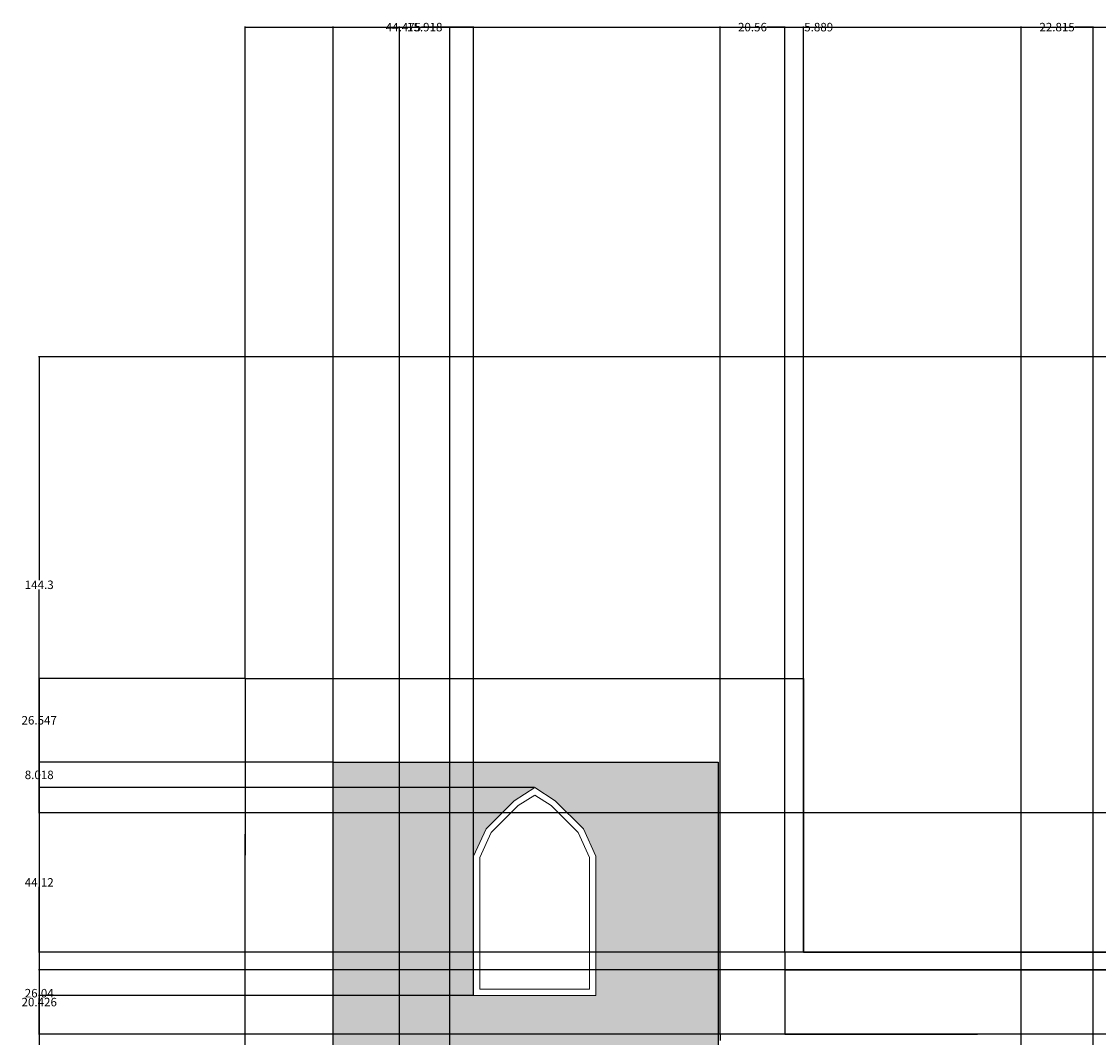
# Model space of a CAD drawing. Units: inches. Extents: x 2 to 1442, y 20 to 729.
# Tile 2 of 8: x 2 to 343, y 407 to 729. Entities that reach past the tile are written whole.
import ezdxf

# ---------------------------------------------------------------- set-up
doc = ezdxf.new("R2010")
doc.units = ezdxf.units.IN
doc.header["$MEASUREMENT"] = 0
for name, color, linetype, lineweight in [('A-ANNO-DIMS', 2, 'Continuous', 18), ('A-ELEV', 7, 'Continuous', 25), ('A-GLAZ', 4, 'Continuous', 18), ('A-WALL-PATT', 8, 'Continuous', 13)]:
    doc.layers.add(name, color=color, linetype=linetype, lineweight=lineweight)
doc.styles.get("Standard").update_dxf_attribs({"font": 'arial.ttf'})
doc.dimstyles.get("Standard").update_dxf_attribs({"dimtxt": 2.6875, "dimasz": 0.18, "dimexe": 0.18, "dimexo": 0.0625, "dimgap": 0.09, "dimtad": 0, "dimtih": 1, "dimtoh": 1, "dimdec": 4, "dimzin": 0, "dimdsep": 46, "dimlunit": 4, "dimtxsty": 'Standard', "dimcen": 0.09, "dimadec": 0, "dimazin": 0, "dimtfac": 1, "dimtdec": 4, "dimtofl": 0, "dimtmove": 0, "dimatfit": 3, "dimfxl": 1, "dimtolj": 1, "dimtzin": 0, "dimarcsym": 0})

# ---------------------------------------------------------------- blocks, each defined once
blk = doc.blocks.new('WIN-ARCH-SMALL')
for points in [[(0, 44.18), (3.93, 52.78), (12.87, 61.71), (19.37, 65.87)], [(38.74, 44.18), (34.82, 52.78), (25.87, 61.71), (19.37, 65.87)], [(2, 43.74), (5.6, 51.62), (14.13, 60.14), (19.37, 63.49)], [(36.74, 43.74), (33.15, 51.62), (24.61, 60.14), (19.37, 63.49)], [(0, 44.18), (0, 0), (38.74, 0), (38.74, 44.18)], [(2, 43.74), (2, 2), (36.74, 2), (36.74, 43.74)]]:
    blk.add_lwpolyline(points)
blk = doc.blocks.new('*D31')
at = {"layer": 'A-ANNO-DIMS', "color": 0, "lineweight": -2, "transparency": 16777216}
for p, q in [((243.46, 433.99), (243.46, 726.93)), ((243.64, 726.75), (249.17, 726.75)), ((249.35, 433.99), (249.35, 726.93)), ((249.35, 726.75), (249.53, 726.75))]:
    blk.add_line(p, q, dxfattribs=at)
at = {"layer": 'A-ANNO-DIMS', "color": 0, "transparency": 16777216}
for points in [[(243.64, 726.78), (243.64, 726.72), (243.46, 726.75)], [(249.17, 726.78), (249.17, 726.72), (249.35, 726.75)]]:
    blk.add_solid(points, dxfattribs=at)
at = {"layer": 'Defpoints', "color": 0, "transparency": 16777216}
for p in [(249.35, 726.75), (243.46, 433.93), (249.35, 433.93)]:
    blk.add_point(p, dxfattribs=at)
at = {"layer": 'A-ANNO-DIMS', "color": 0, "transparency": 16777216, "insert": (254.15, 726.75), "char_height": 2.688, "attachment_point": 5}
blk.add_mtext('\\A1;5.889', dxfattribs=at)
blk = doc.blocks.new('*D32')
at = {"layer": 'A-ANNO-DIMS', "color": 0, "lineweight": -2, "transparency": 16777216}
for p, q in [((72.46, 520.58), (7.1, 520.58)), ((7.28, 520.4), (7.28, 305.39)), ((7.28, 87.45), (7.28, 302.46)), ((72.46, 87.27), (7.1, 87.27))]:
    blk.add_line(p, q, dxfattribs=at)
at = {"layer": 'A-ANNO-DIMS', "color": 0, "transparency": 16777216}
for points in [[(7.25, 520.4), (7.31, 520.4), (7.28, 520.58)], [(7.25, 87.45), (7.31, 87.45), (7.28, 87.27)]]:
    blk.add_solid(points, dxfattribs=at)
at = {"layer": 'Defpoints', "color": 0, "transparency": 16777216}
for p in [(7.28, 520.58), (72.53, 520.58), (72.53, 87.27)]:
    blk.add_point(p, dxfattribs=at)
at = {"layer": 'A-ANNO-DIMS', "color": 0, "transparency": 16777216, "insert": (7.28, 303.93), "char_height": 2.688, "attachment_point": 5}
blk.add_mtext('\\A1;433.3', dxfattribs=at)
blk = doc.blocks.new('*D37')
at = {"layer": 'A-ANNO-DIMS', "color": 0, "lineweight": -2, "transparency": 16777216}
for p, q in [((144.79, 420.15), (7.1, 420.15)), ((7.28, 419.97), (7.28, 388.26)), ((7.28, 353.62), (7.28, 385.33)), ((163.84, 353.44), (7.1, 353.44))]:
    blk.add_line(p, q, dxfattribs=at)
at = {"layer": 'A-ANNO-DIMS', "color": 0, "transparency": 16777216}
for points in [[(7.25, 419.97), (7.31, 419.97), (7.28, 420.15)], [(7.25, 353.62), (7.31, 353.62), (7.28, 353.44)]]:
    blk.add_solid(points, dxfattribs=at)
at = {"layer": 'Defpoints', "color": 0, "transparency": 16777216}
for p in [(7.28, 420.15), (144.86, 420.15), (163.9, 353.44)]:
    blk.add_point(p, dxfattribs=at)
at = {"layer": 'A-ANNO-DIMS', "color": 0, "transparency": 16777216, "insert": (7.28, 386.79), "char_height": 2.688, "attachment_point": 5}
blk.add_mtext('\\A1;66.71', dxfattribs=at)
blk = doc.blocks.new('*D38')
at = {"layer": 'A-ANNO-DIMS', "color": 0, "lineweight": -2, "transparency": 16777216}
for p, q in [((100.32, 494.04), (7.1, 494.04)), ((7.28, 493.86), (7.28, 491.49)), ((7.28, 486.2), (7.28, 488.56)), ((164.17, 486.02), (7.1, 486.02))]:
    blk.add_line(p, q, dxfattribs=at)
at = {"layer": 'A-ANNO-DIMS', "color": 0, "transparency": 16777216}
for points in [[(7.25, 493.86), (7.31, 493.86), (7.28, 494.04)], [(7.25, 486.2), (7.31, 486.2), (7.28, 486.02)]]:
    blk.add_solid(points, dxfattribs=at)
at = {"layer": 'Defpoints', "color": 0, "transparency": 16777216}
for p in [(7.28, 494.04), (100.38, 494.04), (164.23, 486.02)]:
    blk.add_point(p, dxfattribs=at)
at = {"layer": 'A-ANNO-DIMS', "color": 0, "transparency": 16777216, "insert": (7.28, 490.03), "char_height": 2.688, "attachment_point": 5}
blk.add_mtext('\\A1;8.018', dxfattribs=at)
blk = doc.blocks.new('*D39')
at = {"layer": 'A-ANNO-DIMS', "color": 0, "lineweight": -2, "transparency": 16777216}
for p, q in [((72.46, 520.58), (7.1, 520.58)), ((7.28, 520.4), (7.28, 508.77)), ((7.28, 494.22), (7.28, 505.85)), ((100.32, 494.04), (7.1, 494.04))]:
    blk.add_line(p, q, dxfattribs=at)
at = {"layer": 'A-ANNO-DIMS', "color": 0, "transparency": 16777216}
for points in [[(7.25, 520.4), (7.31, 520.4), (7.28, 520.58)], [(7.25, 494.22), (7.31, 494.22), (7.28, 494.04)]]:
    blk.add_solid(points, dxfattribs=at)
at = {"layer": 'Defpoints', "color": 0, "transparency": 16777216}
for p in [(7.28, 520.58), (72.53, 520.58), (100.38, 494.04)]:
    blk.add_point(p, dxfattribs=at)
at = {"layer": 'A-ANNO-DIMS', "color": 0, "transparency": 16777216, "insert": (7.28, 507.31), "char_height": 2.688, "attachment_point": 5}
blk.add_mtext('\\A1;26.547', dxfattribs=at)
blk = doc.blocks.new('*D40')
at = {"layer": 'A-ANNO-DIMS', "color": 0, "lineweight": -2, "transparency": 16777216}
for p, q in [((100.38, 494.1), (100.38, 726.93)), ((100.56, 726.75), (116.89, 726.75)), ((144.68, 726.75), (128.35, 726.75)), ((144.86, 420.21), (144.86, 726.93))]:
    blk.add_line(p, q, dxfattribs=at)
at = {"layer": 'A-ANNO-DIMS', "color": 0, "transparency": 16777216}
for points in [[(100.56, 726.78), (100.56, 726.72), (100.38, 726.75)], [(144.68, 726.78), (144.68, 726.72), (144.86, 726.75)]]:
    blk.add_solid(points, dxfattribs=at)
at = {"layer": 'Defpoints', "color": 0, "transparency": 16777216}
for p in [(144.86, 726.75), (100.38, 494.04), (144.86, 420.15)]:
    blk.add_point(p, dxfattribs=at)
at = {"layer": 'A-ANNO-DIMS', "color": 0, "transparency": 16777216, "insert": (122.62, 726.75), "char_height": 2.688, "attachment_point": 5}
blk.add_mtext('\\A1;44.475', dxfattribs=at)
blk = doc.blocks.new('*D42')
at = {"layer": 'A-ANNO-DIMS', "color": 0, "lineweight": -2, "transparency": 16777216}
for p, q in [((121.42, 97.68), (121.42, 726.93)), ((121.6, 726.75), (123.84, 726.75)), ((137.16, 726.75), (134.93, 726.75)), ((137.34, 97.68), (137.34, 726.93))]:
    blk.add_line(p, q, dxfattribs=at)
at = {"layer": 'A-ANNO-DIMS', "color": 0, "transparency": 16777216}
for points in [[(121.6, 726.78), (121.6, 726.72), (121.42, 726.75)], [(137.16, 726.78), (137.16, 726.72), (137.34, 726.75)]]:
    blk.add_solid(points, dxfattribs=at)
at = {"layer": 'Defpoints', "color": 0, "transparency": 16777216}
for p in [(137.34, 726.75), (121.42, 97.62), (137.34, 97.62)]:
    blk.add_point(p, dxfattribs=at)
at = {"layer": 'A-ANNO-DIMS', "color": 0, "transparency": 16777216, "insert": (129.38, 726.75), "char_height": 2.688, "attachment_point": 5}
blk.add_mtext('\\A1;15.918', dxfattribs=at)
blk = doc.blocks.new('*D43')
at = {"layer": 'A-ANNO-DIMS', "color": 0, "lineweight": -2, "transparency": 16777216}
for p, q in [((222.84, 407.89), (7.1, 407.89)), ((7.28, 407.71), (7.28, 249.04)), ((7.28, 87.45), (7.28, 246.12)), ((232.22, 87.27), (7.1, 87.27))]:
    blk.add_line(p, q, dxfattribs=at)
at = {"layer": 'A-ANNO-DIMS', "color": 0, "transparency": 16777216}
for points in [[(7.25, 407.71), (7.31, 407.71), (7.28, 407.89)], [(7.25, 87.45), (7.31, 87.45), (7.28, 87.27)]]:
    blk.add_solid(points, dxfattribs=at)
at = {"layer": 'Defpoints', "color": 0, "transparency": 16777216}
for p in [(7.28, 407.89), (222.9, 407.89), (232.28, 87.27)]:
    blk.add_point(p, dxfattribs=at)
at = {"layer": 'A-ANNO-DIMS', "color": 0, "transparency": 16777216, "insert": (7.28, 247.58), "char_height": 2.688, "attachment_point": 5}
blk.add_mtext('\\A1;320.6', dxfattribs=at)
blk = doc.blocks.new('*D44')
at = {"layer": 'A-ANNO-DIMS', "color": 0, "lineweight": -2, "transparency": 16777216}
for p, q in [((243.4, 433.93), (7.1, 433.93)), ((7.28, 433.75), (7.28, 422.37)), ((7.28, 408.07), (7.28, 419.44)), ((222.84, 407.89), (7.1, 407.89))]:
    blk.add_line(p, q, dxfattribs=at)
at = {"layer": 'A-ANNO-DIMS', "color": 0, "transparency": 16777216}
for points in [[(7.25, 433.75), (7.31, 433.75), (7.28, 433.93)], [(7.25, 408.07), (7.31, 408.07), (7.28, 407.89)]]:
    blk.add_solid(points, dxfattribs=at)
at = {"layer": 'Defpoints', "color": 0, "transparency": 16777216}
for p in [(243.46, 433.93), (7.28, 407.89), (222.9, 407.89)]:
    blk.add_point(p, dxfattribs=at)
at = {"layer": 'A-ANNO-DIMS', "color": 0, "transparency": 16777216, "insert": (7.28, 420.91), "char_height": 2.688, "attachment_point": 5}
blk.add_mtext('\\A1;26.04', dxfattribs=at)
blk = doc.blocks.new('*D45')
at = {"layer": 'A-ANNO-DIMS', "color": 0, "lineweight": -2, "transparency": 16777216}
for p, q in [((222.9, 407.95), (222.9, 726.93)), ((223.08, 726.75), (228.53, 726.75)), ((243.28, 726.75), (237.83, 726.75)), ((243.46, 433.99), (243.46, 726.93))]:
    blk.add_line(p, q, dxfattribs=at)
at = {"layer": 'A-ANNO-DIMS', "color": 0, "transparency": 16777216}
for points in [[(223.08, 726.78), (223.08, 726.72), (222.9, 726.75)], [(243.28, 726.78), (243.28, 726.72), (243.46, 726.75)]]:
    blk.add_solid(points, dxfattribs=at)
at = {"layer": 'Defpoints', "color": 0, "transparency": 16777216}
for p in [(243.46, 726.75), (243.46, 433.93), (222.9, 407.89)]:
    blk.add_point(p, dxfattribs=at)
at = {"layer": 'A-ANNO-DIMS', "color": 0, "transparency": 16777216, "insert": (233.18, 726.75), "char_height": 2.688, "attachment_point": 5}
blk.add_mtext('\\A1;20.56', dxfattribs=at)
blk = doc.blocks.new('*D47')
at = {"layer": 'A-ANNO-DIMS', "color": 0, "lineweight": -2, "transparency": 16777216}
for p, q in [((318.25, 215.98), (318.25, 726.93)), ((318.43, 726.75), (323.95, 726.75)), ((340.88, 726.75), (335.36, 726.75)), ((341.06, 215.98), (341.06, 726.93))]:
    blk.add_line(p, q, dxfattribs=at)
at = {"layer": 'A-ANNO-DIMS', "color": 0, "transparency": 16777216}
for points in [[(318.43, 726.78), (318.43, 726.72), (318.25, 726.75)], [(340.88, 726.78), (340.88, 726.72), (341.06, 726.75)]]:
    blk.add_solid(points, dxfattribs=at)
at = {"layer": 'Defpoints', "color": 0, "transparency": 16777216}
for p in [(341.06, 726.75), (318.25, 215.92), (341.06, 215.92)]:
    blk.add_point(p, dxfattribs=at)
at = {"layer": 'A-ANNO-DIMS', "color": 0, "transparency": 16777216, "insert": (329.65, 726.75), "char_height": 2.688, "attachment_point": 5}
blk.add_mtext('\\A1;22.815', dxfattribs=at)
blk = doc.blocks.new('*D61')
at = {"layer": 'A-ANNO-DIMS', "color": 0, "lineweight": -2, "transparency": 16777216}
for p, q in [((432.9, 428.31), (7.1, 428.31)), ((7.28, 428.13), (7.28, 419.56)), ((7.28, 408.07), (7.28, 416.64)), ((432.9, 407.89), (7.1, 407.89))]:
    blk.add_line(p, q, dxfattribs=at)
at = {"layer": 'A-ANNO-DIMS', "color": 0, "transparency": 16777216}
for points in [[(7.25, 428.13), (7.31, 428.13), (7.28, 428.31)], [(7.25, 408.07), (7.31, 408.07), (7.28, 407.89)]]:
    blk.add_solid(points, dxfattribs=at)
at = {"layer": 'Defpoints', "color": 0, "transparency": 16777216}
for p in [(7.28, 428.31), (432.97, 428.31), (432.97, 407.89)]:
    blk.add_point(p, dxfattribs=at)
at = {"layer": 'A-ANNO-DIMS', "color": 0, "transparency": 16777216, "insert": (7.28, 418.1), "char_height": 2.688, "attachment_point": 5}
blk.add_mtext('\\A1;20.426', dxfattribs=at)
blk = doc.blocks.new('*D68')
at = {"layer": 'A-ANNO-DIMS', "color": 0, "lineweight": -2, "transparency": 16777216}
for p, q in [((721.76, 622.36), (7.1, 622.36)), ((7.28, 622.18), (7.28, 551.67)), ((7.28, 478.23), (7.28, 548.74)), ((590.13, 478.05), (7.1, 478.05))]:
    blk.add_line(p, q, dxfattribs=at)
at = {"layer": 'A-ANNO-DIMS', "color": 0, "transparency": 16777216}
for points in [[(7.25, 622.18), (7.31, 622.18), (7.28, 622.36)], [(7.25, 478.23), (7.31, 478.23), (7.28, 478.05)]]:
    blk.add_solid(points, dxfattribs=at)
at = {"layer": 'Defpoints', "color": 0, "transparency": 16777216}
for p in [(7.28, 622.36), (721.83, 622.36), (590.19, 478.05)]:
    blk.add_point(p, dxfattribs=at)
at = {"layer": 'A-ANNO-DIMS', "color": 0, "transparency": 16777216, "insert": (7.28, 550.2), "char_height": 2.688, "attachment_point": 5}
blk.add_mtext('\\A1;144.3', dxfattribs=at)
blk = doc.blocks.new('*D69')
at = {"layer": 'A-ANNO-DIMS', "color": 0, "lineweight": -2, "transparency": 16777216}
for p, q in [((590.13, 478.05), (7.1, 478.05)), ((7.28, 477.87), (7.28, 457.43)), ((7.28, 434.11), (7.28, 454.55)), ((549, 433.93), (7.1, 433.93))]:
    blk.add_line(p, q, dxfattribs=at)
at = {"layer": 'A-ANNO-DIMS', "color": 0, "transparency": 16777216}
for points in [[(7.25, 477.87), (7.31, 477.87), (7.28, 478.05)], [(7.25, 434.11), (7.31, 434.11), (7.28, 433.93)]]:
    blk.add_solid(points, dxfattribs=at)
at = {"layer": 'Defpoints', "color": 0, "transparency": 16777216}
for p in [(7.28, 478.05), (590.19, 478.05), (549.07, 433.93)]:
    blk.add_point(p, dxfattribs=at)
at = {"layer": 'A-ANNO-DIMS', "color": 0, "transparency": 16777216, "insert": (7.28, 455.99), "char_height": 2.688, "attachment_point": 5}
blk.add_mtext('\\A1;44.12', dxfattribs=at)
blk = doc.blocks.new('*D82')
at = {"layer": 'A-ANNO-DIMS', "color": 0, "lineweight": -2, "transparency": 16777216}
for p, q in [((72.53, 520.64), (72.53, 726.93)), ((72.71, 726.75), (716.28, 726.75)), ((1370.94, 726.75), (727.37, 726.75)), ((1371.12, 520.64), (1371.12, 726.93))]:
    blk.add_line(p, q, dxfattribs=at)
at = {"layer": 'A-ANNO-DIMS', "color": 0, "transparency": 16777216}
for points in [[(72.71, 726.78), (72.71, 726.72), (72.53, 726.75)], [(1370.94, 726.78), (1370.94, 726.72), (1371.12, 726.75)]]:
    blk.add_solid(points, dxfattribs=at)
at = {"layer": 'Defpoints', "color": 0, "transparency": 16777216}
for p in [(1371.12, 726.75), (72.53, 520.58), (1371.12, 520.58)]:
    blk.add_point(p, dxfattribs=at)
at = {"layer": 'A-ANNO-DIMS', "color": 0, "transparency": 16777216, "insert": (721.83, 726.75), "char_height": 2.688, "attachment_point": 5}
blk.add_mtext('\\A1;1298.6', dxfattribs=at)

msp = doc.modelspace()

# ---------------------------------------------------------------- hatches: boundary and pattern name
at = {"layer": 'A-WALL-PATT'}
h = msp.add_hatch(dxfattribs=at)
h.set_pattern_fill('BRASS', color=256, scale=14)
h.paths.add_polyline_path([(222.3553, 494.0357), (100.382, 494.0357), (100.382, 87.2714), (118.4234, 87.2714), (118.4234, 261.6116), (130.3451, 261.6116), (130.3451, 275.7919), (130.3451, 320.992), (130.3451, 322.0535), (130.6686, 323.8227), (133.191, 330.4901), (134.3119, 332.5101), (138.9535, 338.5974), (142.6478, 343.4423), (143.8105, 344.5736), (150.3377, 349.2734), (151.6201, 349.9601), (160.0334, 353.1203), (161.7915, 353.4396), (163.9013, 353.4396), (165.6594, 353.1203), (174.0727, 349.9601), (175.3551, 349.2734), (181.8823, 344.5736), (183.045, 343.4423), (186.7393, 338.5974), (191.601, 332.2216), (192.3734, 330.8295), (195.0242, 323.8227), (195.3477, 322.0535), (195.3477, 320.992), (195.3477, 276.0187), (195.3477, 261.5562), (207.2798, 261.5562), (207.2798, 87.2714), (222.3553, 87.2714)])
h.paths.add_polyline_path([(144.8571, 420.1495), (144.8571, 464.3282), (148.784, 472.9254), (157.7288, 481.8631), (164.2287, 486.0178), (170.7285, 481.8631), (179.6733, 472.9254), (183.6002, 464.3282), (183.6002, 420.1495)], flags=16)
h.paths.add_polyline_path([(146.8571, 422.1495), (146.8571, 463.893), (150.4531, 471.7659), (158.9889, 480.2948), (164.2287, 483.6441), (169.4684, 480.2948), (178.0042, 471.7659), (181.6002, 463.893), (181.6002, 422.1495)], flags=0)

# ---------------------------------------------------------------- linework, layer by layer
at = {"layer": 'A-ELEV'}
for p, q in [((72.5272, 520.5823), (249.3478, 520.5823)), ((72.5272, 520.5823), (72.5272, 464.6214)), ((249.3478, 520.5823), (249.3478, 471.2714)), ((72.5272, 423.2714), (72.5272, 471.2714)), ((249.3478, 471.2714), (249.3478, 433.9259)), ((245.2684, 433.9259), (243.4592, 433.9259)), ((243.4592, 433.9259), (243.4592, 422.7015)), ((249.3478, 433.9259), (245.2684, 433.9259)), ((249.3478, 433.9259), (405.1329, 433.9259)), ((243.4592, 428.3137), (405.2452, 428.3137)), ((72.5272, 255.2714), (72.5272, 423.2714)), ((243.4592, 422.7015), (243.4592, 407.8873)), ((243.4592, 407.8873), (222.8994, 407.8873)), ((222.8994, 407.8873), (222.8994, 405.9114)), ((243.4592, 407.8873), (249.3478, 407.8873)), ((249.3478, 407.8873), (291.5616, 407.8873)), ((291.5616, 407.8873), (304.4461, 407.8873)), ((344.4513, 407.8873), (304.4461, 407.8873))]:
    msp.add_line(p, q, dxfattribs=at)
msp.add_lwpolyline([(100.382, 494.0357), (222.3553, 494.0357), (222.3553, 87.2714), (100.382, 87.2714)], close=True, dxfattribs=at)

# ---------------------------------------------------------------- block references
at = {"layer": 'A-GLAZ'}
msp.add_blockref('WIN-ARCH-SMALL', (144.857, 420.15), dxfattribs=at)

# ---------------------------------------------------------------- dimensions: what is measured, and where the dimension line sits
at = {"layer": 'A-ANNO-DIMS'}
for base, p1, p2, override, picture, middle in [((1371.1242, 726.75), (72.5272, 520.5823), (1371.1242, 520.5823), {"dimdec": 1, "dimlfac": 1, "dimrnd": 0, "dimzin": 0, "dimdsep": 46, "dimlunit": 2}, '*D82', (721.8257, 726.75)), ((144.8571, 726.75), (100.382, 494.0357), (144.8571, 420.1495), {"dimdec": 3, "dimlfac": 1, "dimrnd": 0, "dimzin": 0, "dimdsep": 46, "dimlunit": 2}, '*D40', (122.6196, 726.75)), ((137.3412, 726.75), (121.4234, 97.6222), (137.3412, 97.6222), {"dimdec": 3, "dimlfac": 1, "dimrnd": 0, "dimzin": 0, "dimdsep": 46, "dimlunit": 2}, '*D42', (129.3823, 726.75)), ((243.4592, 726.75), (222.8994, 407.8873), (243.4592, 433.9259), {"dimdec": 2, "dimlfac": 1, "dimrnd": 0, "dimzin": 0, "dimdsep": 46, "dimlunit": 2}, '*D45', (233.1793, 726.75)), ((249.3478, 726.75), (243.4592, 433.9259), (249.3478, 433.9259), {"dimdec": 3, "dimlfac": 1, "dimrnd": 0, "dimzin": 0, "dimdsep": 46, "dimlunit": 2}, '*D31', (254.155, 726.75)), ((341.0623, 726.75), (318.2474, 215.9163), (341.0623, 215.9163), {"dimdec": 3, "dimlfac": 1, "dimrnd": 0, "dimzin": 0, "dimdsep": 46, "dimlunit": 2}, '*D47', (329.6548, 726.75))]:
    dim = msp.add_linear_dim(base=base, p1=p1, p2=p2, dimstyle='Standard', override=override, dxfattribs=at)
    dim.commit()
    dim.dimension.update_dxf_attribs({"geometry": picture, "text_midpoint": middle})
for base, p1, p2, override, picture, middle in [((7.2772, 622.3576), (590.1914, 478.0502), (721.8257, 622.3576), {"dimdec": 1, "dimlfac": 1, "dimrnd": 0, "dimzin": 0, "dimdsep": 46, "dimlunit": 2}, '*D68', (7.2772, 550.2039)), ((7.2772, 520.5823), (100.382, 494.0357), (72.5272, 520.5823), {"dimdec": 3, "dimlfac": 1, "dimrnd": 0, "dimzin": 0, "dimdsep": 46, "dimlunit": 2}, '*D39', (7.2772, 507.309)), ((7.2772, 520.5823), (72.5272, 87.2714), (72.5272, 520.5823), {"dimdec": 1, "dimlfac": 1, "dimrnd": 0, "dimzin": 0, "dimdsep": 46, "dimlunit": 2}, '*D32', (7.2772, 303.9269)), ((7.2772, 494.0357), (164.2287, 486.0178), (100.382, 494.0357), {"dimdec": 3, "dimlfac": 1, "dimrnd": 0, "dimzin": 0, "dimdsep": 46, "dimlunit": 2}, '*D38', (7.2772, 490.0267)), ((7.2772, 478.0502), (549.0669, 433.9259), (590.1914, 478.0502), {"dimdec": 2, "dimlfac": 1, "dimrnd": 0, "dimzin": 0, "dimdsep": 46, "dimlunit": 2}, '*D69', (7.2772, 455.9881)), ((7.2772, 407.8873), (243.4592, 433.9259), (222.8994, 407.8873), {"dimdec": 2, "dimlfac": 1, "dimrnd": 0, "dimzin": 0, "dimdsep": 46, "dimlunit": 2}, '*D44', (7.2772, 420.9066)), ((7.2772, 428.3137), (432.9658, 407.8873), (432.9658, 428.3137), {"dimdec": 3, "dimlfac": 1, "dimrnd": 0, "dimzin": 0, "dimdsep": 46, "dimlunit": 2}, '*D61', (7.2772, 418.1005)), ((7.2772, 420.1495), (163.9013, 353.4396), (144.8571, 420.1495), {"dimdec": 2, "dimlfac": 1, "dimrnd": 0, "dimzin": 0, "dimdsep": 46, "dimlunit": 2}, '*D37', (7.2772, 386.7945)), ((7.2772, 407.8873), (232.2824, 87.2714), (222.8994, 407.8873), {"dimdec": 1, "dimlfac": 1, "dimrnd": 0, "dimzin": 0, "dimdsep": 46, "dimlunit": 2}, '*D43', (7.2772, 247.5793))]:
    dim = msp.add_linear_dim(base=base, p1=p1, p2=p2, angle=90, dimstyle='Standard', override=override, dxfattribs=at)
    dim.commit()
    dim.dimension.update_dxf_attribs({"geometry": picture, "text_midpoint": middle})

doc.saveas('drawing.dxf')
